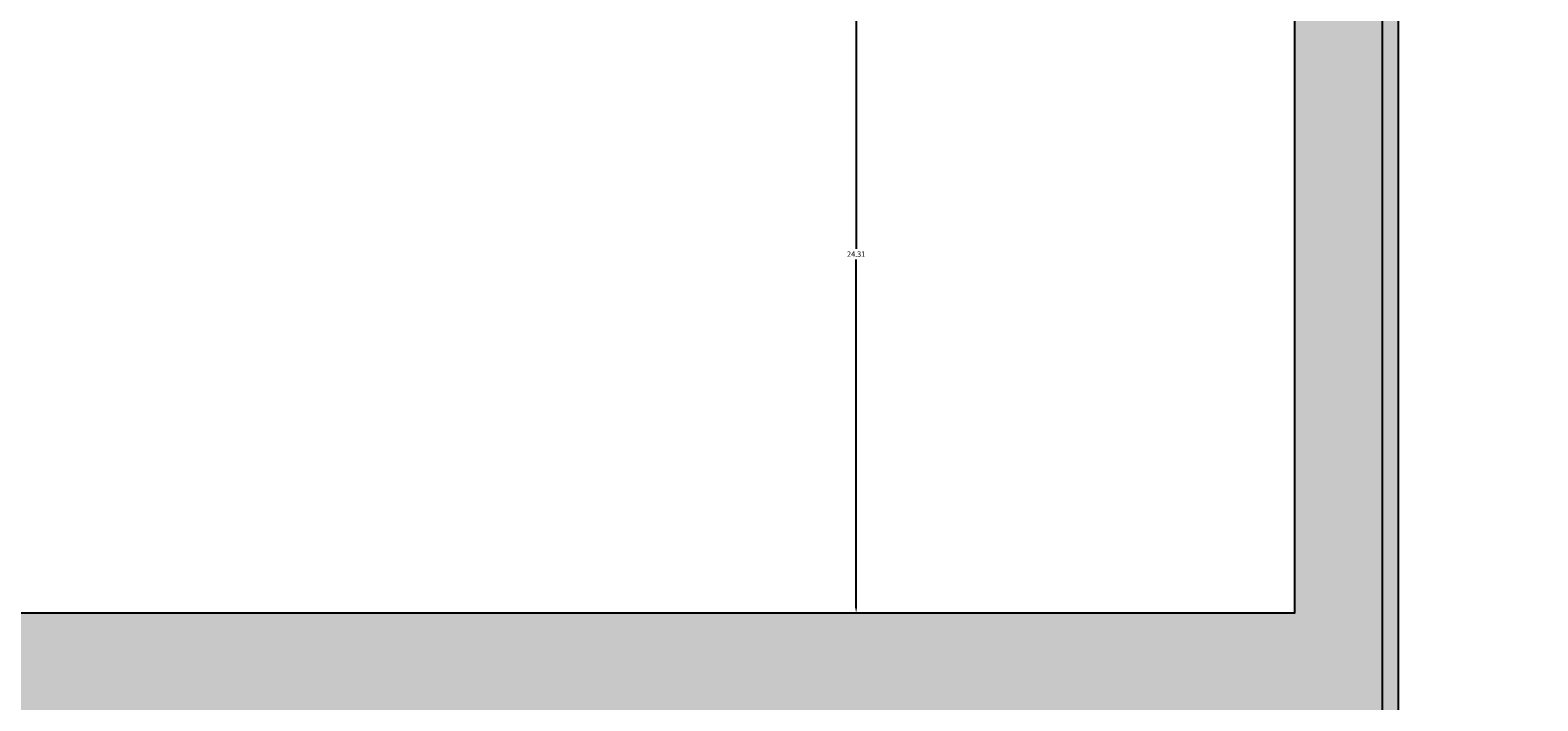
# Model space of a CAD drawing. Units: millimetres. Extents: x -11 to 280, y -4 to 208.
# Tile 48 of 55: x 186 to 237, y 106 to 129. Entities that reach past the tile are written whole.
import ezdxf

# ---------------------------------------------------------------- set-up
doc = ezdxf.new("R2010")
doc.units = ezdxf.units.MM
doc.layers.add('M-DIMS', color=2, linetype='Continuous', lineweight=18)
doc.layers.add('M-HYDR-PRES', color=7, linetype='Continuous', lineweight=25)
doc.layers.add('M-HYDR-PRES-PATT', color=240, linetype='Continuous', lineweight=13, true_color=0xed1f24)
doc.styles.get("Standard").update_dxf_attribs({"font": 'arial.ttf'})
doc.dimstyles.get("Standard").update_dxf_attribs({"dimtxt": 0.18, "dimasz": 0.18, "dimexe": 0.18, "dimexo": 0.0625, "dimgap": 0.09, "dimtad": 0, "dimtih": 1, "dimtoh": 1, "dimdec": 4, "dimzin": 0, "dimdsep": 46, "dimtxsty": 'Standard', "dimcen": 0.09, "dimadec": 0, "dimazin": 0, "dimtfac": 1, "dimtdec": 4, "dimtofl": 0, "dimtmove": 0, "dimatfit": 3, "dimfxl": 1, "dimtolj": 1, "dimtzin": 0, "dimarcsym": 0})

# ---------------------------------------------------------------- blocks, each defined once
blk = doc.blocks.new('*D5')
at = {"layer": 'Defpoints', "color": 0, "transparency": 16777216}
for p in [(24.759, 192.645), (-10.087, 11.435), (261.686, 11.435)]:
    blk.add_point(p, dxfattribs=at)
at = {"layer": 'M-DIMS', "color": 0, "lineweight": -2, "transparency": 16777216}
for p, q in [((24.696, 192.645), (-10.267, 192.645)), ((-10.087, 192.465), (-10.087, 102.222)), ((-10.087, 11.615), (-10.087, 101.858)), ((261.624, 11.435), (-10.267, 11.435))]:
    blk.add_line(p, q, dxfattribs=at)
at = {"layer": 'M-DIMS', "color": 0, "transparency": 16777216}
for points in [[(-10.117, 192.465), (-10.057, 192.465), (-10.087, 192.645)], [(-10.117, 11.615), (-10.057, 11.615), (-10.087, 11.435)]]:
    blk.add_solid(points, dxfattribs=at)
at = {"layer": 'M-DIMS', "color": 0, "transparency": 16777216, "insert": (-10.087, 102.04), "char_height": 0.18, "attachment_point": 5}
blk.add_mtext('\\A1;181.2', dxfattribs=at)
blk = doc.blocks.new('*D15')
at = {"layer": 'Defpoints', "color": 0, "transparency": 16777216}
for p in [(213.85, 133.123), (228.7, 133.123), (228.7, 108.814)]:
    blk.add_point(p, dxfattribs=at)
at = {"layer": 'M-DIMS', "color": 0, "lineweight": -2, "transparency": 16777216}
for p, q in [((228.638, 133.123), (213.67, 133.123)), ((213.85, 132.943), (213.85, 121.15)), ((213.85, 108.994), (213.85, 120.786)), ((228.638, 108.814), (213.67, 108.814))]:
    blk.add_line(p, q, dxfattribs=at)
at = {"layer": 'M-DIMS', "color": 0, "transparency": 16777216}
for points in [[(213.82, 132.943), (213.88, 132.943), (213.85, 133.123)], [(213.82, 108.994), (213.88, 108.994), (213.85, 108.814)]]:
    blk.add_solid(points, dxfattribs=at)
at = {"layer": 'M-DIMS', "color": 0, "transparency": 16777216, "insert": (213.85, 120.968), "char_height": 0.18, "attachment_point": 5}
blk.add_mtext('\\A1;24.31', dxfattribs=at)
blk = doc.blocks.new('*D20')
at = {"layer": 'Defpoints', "color": 0, "transparency": 16777216}
for p in [(231.68, 207.495), (151.022, 43.599), (231.68, 43.599)]:
    blk.add_point(p, dxfattribs=at)
at = {"layer": 'M-DIMS', "color": 0, "lineweight": -2, "transparency": 16777216}
for p, q in [((151.022, 43.662), (151.022, 207.675)), ((151.202, 207.495), (190.957, 207.495)), ((231.5, 207.495), (191.745, 207.495)), ((231.68, 43.662), (231.68, 207.675))]:
    blk.add_line(p, q, dxfattribs=at)
at = {"layer": 'M-DIMS', "color": 0, "transparency": 16777216}
for points in [[(151.202, 207.525), (151.202, 207.465), (151.022, 207.495)], [(231.5, 207.525), (231.5, 207.465), (231.68, 207.495)]]:
    blk.add_solid(points, dxfattribs=at)
at = {"layer": 'M-DIMS', "color": 0, "transparency": 16777216, "insert": (191.351, 207.495), "char_height": 0.18, "attachment_point": 5}
blk.add_mtext('\\A1;80.66', dxfattribs=at)
blk = doc.blocks.new('*D22')
at = {"layer": 'Defpoints', "color": 0, "transparency": 16777216}
for p in [(259.871, 207.495), (231.68, 34.723), (259.871, 34.723)]:
    blk.add_point(p, dxfattribs=at)
at = {"layer": 'M-DIMS', "color": 0, "lineweight": -2, "transparency": 16777216}
for p, q in [((231.68, 34.785), (231.68, 207.675)), ((231.86, 207.495), (245.38, 207.495)), ((259.691, 207.495), (246.171, 207.495)), ((259.871, 34.785), (259.871, 207.675))]:
    blk.add_line(p, q, dxfattribs=at)
at = {"layer": 'M-DIMS', "color": 0, "transparency": 16777216}
for points in [[(231.86, 207.525), (231.86, 207.465), (231.68, 207.495)], [(259.691, 207.525), (259.691, 207.465), (259.871, 207.495)]]:
    blk.add_solid(points, dxfattribs=at)
at = {"layer": 'M-DIMS', "color": 0, "transparency": 16777216, "insert": (245.776, 207.495), "char_height": 0.18, "attachment_point": 5}
blk.add_mtext('\\A1;28.19', dxfattribs=at)

msp = doc.modelspace()

# ---------------------------------------------------------------- hatches: boundary and pattern name
at = {"layer": 'M-HYDR-PRES-PATT'}
h = msp.add_hatch(color=256, dxfattribs=at)
h.set_gradient(color1=(237, 31, 36), color2=(237, 31, 36), tint=1)
h.paths.add_polyline_path([(232.2, 133.1228), (228.7, 133.1228), (228.7, 108.8141), (102.7646, 108.8141), (102.7646, 105.3141), (232.2, 105.3141)])
h.paths.add_polyline_path([(128.8433, 105.3141), (125.3433, 105.3141), (125.3433, 91.7099, 1), (128.8433, 91.7099)])
h.paths.add_polyline_path([(229.1617, 78.7098), (196.7745, 78.7098, -0.4142136), (191.7745, 83.7098), (191.7745, 105.3141), (188.2745, 105.3141), (188.2745, 80.2098, 0.4142136), (193.2745, 75.2098), (225.6617, 75.2098), (225.6617, 43.5991), (229.1617, 43.5991)])
h.paths.add_polyline_path([(102.7646, 110.3704), (95.5776, 110.3704), (95.5776, 103.9022), (102.7646, 103.9022)])
h.paths.add_polyline_path([(100.7059, 107.2502), (99.1711, 106.3641), (99.1711, 106.8641), (97.1711, 106.8641), (97.1711, 107.6363), (99.1711, 107.6363), (99.1711, 108.1363)], flags=16)
h.paths.add_polyline_path([(234.6119, 138.4081), (226.5106, 138.4081), (226.5106, 133.1228), (234.6119, 133.1228)])
h.paths.add_polyline_path([(231.1963, 135.7055), (230.2965, 134.1786), (229.4241, 135.7213), (229.9241, 135.7168), (229.9418, 137.7167), (230.7141, 137.7099), (230.6963, 135.71)], flags=16)

# ---------------------------------------------------------------- linework, layer by layer
at = {"layer": 'M-HYDR-PRES'}
for points in [[(232.2, 133.1228), (232.2, 105.3141), (102.7646, 105.3141)], [(228.7, 133.1228), (228.7, 108.8141), (102.7646, 108.8141)]]:
    msp.add_lwpolyline(points, dxfattribs=at)

# ---------------------------------------------------------------- dimensions: what is measured, and where the dimension line sits
at = {"layer": 'M-DIMS'}
for base, p1, p2, picture, middle in [((231.6803, 207.495), (151.0217, 43.5991), (231.6803, 43.5991), '*D20', (191.351, 207.495)), ((259.871, 207.495), (231.6803, 34.7226), (259.871, 34.7226), '*D22', (245.7757, 207.495))]:
    dim = msp.add_linear_dim(base=base, p1=p1, p2=p2, dimstyle='Standard', override={"dimdec": 2, "dimlfac": 1, "dimrnd": 0, "dimzin": 0, "dimdsep": 46, "dimlunit": 2}, dxfattribs=at)
    dim.commit()
    dim.dimension.update_dxf_attribs({"geometry": picture, "text_midpoint": middle})
for base, p1, p2, override, picture, middle in [((-10.0865, 11.4346), (24.7588, 192.645), (261.6863, 11.4346), {"dimdec": 1, "dimlfac": 1, "dimrnd": 0, "dimzin": 0, "dimdsep": 46, "dimlunit": 2}, '*D5', (-10.0865, 102.0398)), ((213.85, 133.1228), (228.7, 108.8141), (228.7, 133.1228), {"dimdec": 2, "dimlfac": 1, "dimrnd": 0, "dimzin": 0, "dimdsep": 46, "dimlunit": 2}, '*D15', (213.85, 120.9684))]:
    dim = msp.add_linear_dim(base=base, p1=p1, p2=p2, angle=90, dimstyle='Standard', override=override, dxfattribs=at)
    dim.commit()
    dim.dimension.update_dxf_attribs({"geometry": picture, "text_midpoint": middle})

doc.saveas('drawing.dxf')
